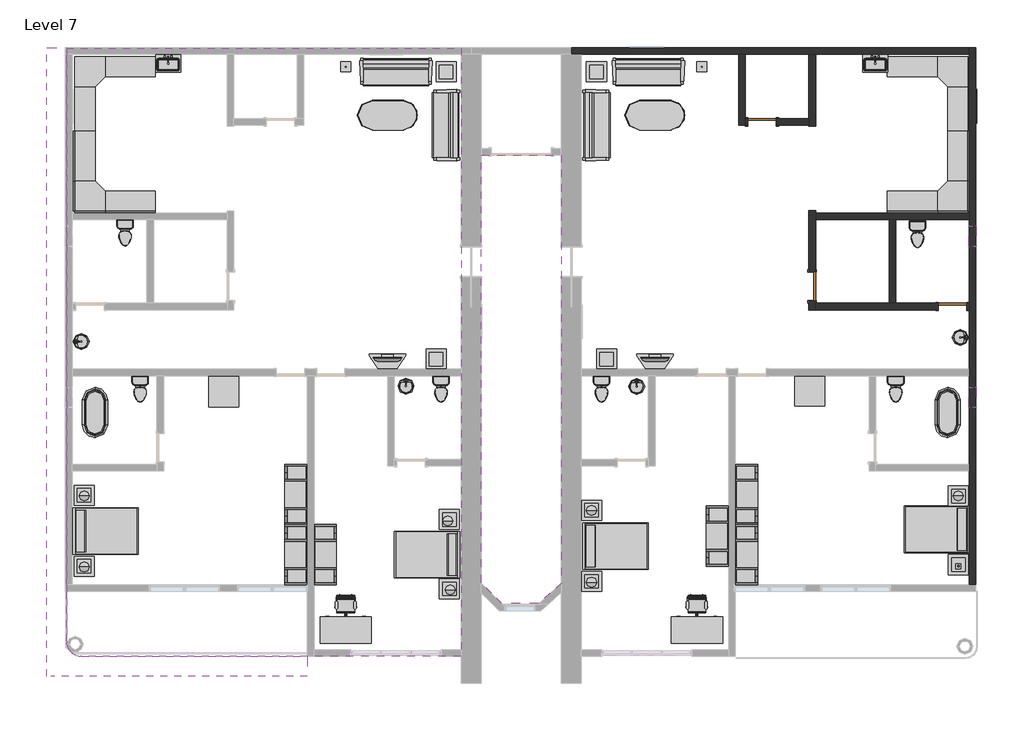
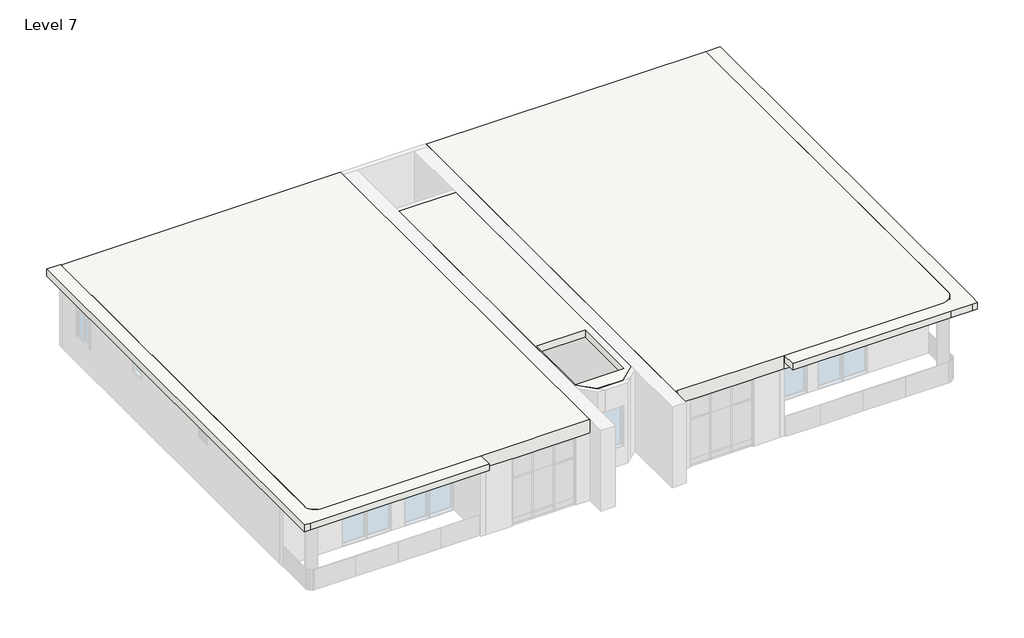
# One storey, part 3 of 3: 42 furniture elements, 14 flow terminals, 10 light fixtures, 9 walls, 3 doors, 3 slabs, 3 windows.
# Revit data of these elements (continued)
# Elements 40, 41 (IfcFurniture, "TV Stand : TV Stand") (continued)
#   Phase Created = New Construction
#   Materials on its faces: "Melamine - Gray", "Glass - Shelves"
# Elements 42, 43, 44, 45, 46, 47, 48, 49, 50, 51, 52, 53 (IfcFurniture, "Table-Coffee : 24\" x 24\" x 24\"")
#   Phase Created = New Construction
#   Materials on its faces: "Glass - Clear, Grey"
# Elements 54, 55 (IfcFurniture, "Table-Dining Oval : 36\" x 72\"")
#   Phase Created = New Construction
#   Materials on its faces: "Steel, Chrome Plated", "Glass - Clear, Grey"
# Elements 56, 57 (IfcFurniture, "Table-Rectangular : 36\" x 36\"")
#   Phase Created = New Construction
#   Materials on its faces: "Birch"
# Elements 58, 59 (IfcFurniture, "Work Station Cubicle : 96\" x 96\"")
#   Phase Created = New Construction
#   Materials on its faces: "Textile - Light Gray", "Laminate, Ivory, Matte"
# Element 60 (IfcLightFixture, "100W - 120V")
#   Mark = "84"
#   Phase Created = New Construction
#   Materials on its faces: "Steel, Chrome Plated", "Glass, Frosted"
# Element 61 (IfcLightFixture, "100W - 120V")
#   Mark = "85"
#   Phase Created = New Construction
#   Materials on its faces: "Steel, Chrome Plated", "Glass, Frosted"
# Element 62 (IfcLightFixture, "Table Lamp - Hemispheric : 60W - 120V")
#   Mark = "86"
#   Phase Created = New Construction
#   Materials on its faces: "Steel, Chrome Plated", "Glass, Frosted", "Birch"
# Element 63 (IfcLightFixture, "Table Lamp - Hemispheric : 60W - 120V")
#   Mark = "87"
#   Phase Created = New Construction
#   Materials on its faces: "Steel, Chrome Plated", "Glass, Frosted", "Birch"
# Element 64 (IfcLightFixture, "Table Lamp - Hemispheric : 60W - 120V")
#   Mark = "88"
#   Phase Created = New Construction
#   Materials on its faces: "Steel, Chrome Plated", "Glass, Frosted", "Birch"
# Element 65 (IfcLightFixture, "Table Lamp - Hemispheric : 60W - 120V")
#   Mark = "89"
#   Phase Created = New Construction
#   Materials on its faces: "Steel, Chrome Plated", "Glass, Frosted", "Birch"
# Element 66 (IfcLightFixture, "Table Lamp - Hemispheric : 60W - 120V")
#   Mark = "90"
#   Phase Created = New Construction
#   Materials on its faces: "Steel, Chrome Plated", "Glass, Frosted", "Birch"
# Element 67 (IfcLightFixture, "Table Lamp - Hemispheric : 60W - 120V")
#   Mark = "91"
#   Phase Created = New Construction
#   Materials on its faces: "Steel, Chrome Plated", "Glass, Frosted", "Birch"
# Element 68 (IfcLightFixture, "Table Lamp - Hemispheric : 60W - 120V")
#   Mark = "92"
#   Phase Created = New Construction
#   Materials on its faces: "Steel, Chrome Plated", "Glass, Frosted", "Birch"
# Element 69 (IfcLightFixture, "Table Lamp - Hemispheric : 60W - 120V")
#   Mark = "93"
#   Phase Created = New Construction
#   Materials on its faces: "Steel, Chrome Plated", "Glass, Frosted", "Birch"
# Element 70 (IfcSlab, "Generic - 12\" cream")
#   Height Offset From Level = 12' - 0"
#   Phase Created = New Construction
#   Materials on its faces: "Parking Stripe"
# Element 71 (IfcSlab, "Generic - 12\" white")
#   built-in parameter 1001955 = 3.14159 (stored number, unit not read)
#   Height Offset From Level = 12' - 0"
#   Phase Created = New Construction
#   Materials on its faces: "Door - Frame"
# Element 72 (IfcSlab, "Generic - 12\" white")
#   Height Offset From Level = 12' - 0"
#   Phase Created = New Construction
#   Materials on its faces: "Door - Frame"
# Elements 73, 74, 75, 76, 77, 78, 79, 80 (IfcWall, "Generic - 8\" cream")
#   Top Offset = 0' - 0"
#   Base Offset = 0' - 0"
#   Unconnected Height = 10' - 0"
#   wall height = 10' - 0"
#   Phase Created = New Construction
#   Base Constraint = Level 7
#   Materials on its faces: "Parking Stripe"
# Element 81 (IfcWall, "Generic - 8\" white")
#   Top Offset = 0' - 0"
#   Base Offset = 0' - 0"
#   Unconnected Height = 10' - 0"
#   wall height = 10' - 0"
#   Phase Created = New Construction
#   Base Constraint = Level 7
#   Materials on its faces: "Door - Frame", "Parking Stripe"
# Element 82 (IfcWindow, "Louvers with Trim : 24\" x 24\"")
#   Mark = "167"
#   Phase Created = New Construction
#   Materials on its faces: "Glass", "Iron, Ductile"
# Element 83 (IfcWindow, "Louvers with Trim : 24\" x 24\"")
#   Mark = "168"
#   Phase Created = New Construction
#   Materials on its faces: "Glass", "Iron, Ductile"
# Element 84 (IfcWindow, "Slider with Trim : 36\" x 48\"")
#   Mark = "164"
#   Phase Created = New Construction
#   Materials on its faces: "Iron, Ductile", "Glass"
# Materials
#   "Wood - Birch - Solid Stained Light Low Gloss": class "Wood", colour RGB 210 159 95, transparency 0, Cost = 0
#   "Paint - Sienna": colour RGB 118 70 51, transparency 0, Cost = 0
#   "Steel, Polished": class "Metal", colour RGB 57 57 57, transparency 0, Description = "Polished steel", Cost = 0
#   "Porcelain, Linen": class "Ceramic", colour RGB 249 239 230, transparency 0, Description = "Porcelain, linen", Cost = 0
#   "Laminate, Linen, Matte": class "Plastic", colour RGB 249 239 230, transparency 0, Description = "Plastic Laminate - Linen, Matte", Cost = 0
#   "Porcelain, Ivory": class "Ceramic", colour RGB 247 247 239, transparency 0, Description = "Porcelain, ivory", Cost = 0
#   "Laminate, Ivory, Matte": class "Plastic", colour RGB 247 247 239, transparency 0, Description = "Plastic Laminate - Ivory, Matte", Cost = 0
#   "Birch": class "Wood", colour RGB 224 178 126, transparency 0, Description = "Betula Alleghaniensis", Cost = 0
#   "Linen, White": class "Textile", colour RGB 247 247 239, transparency 0, Description = "Linen, white", Cost = 0
#   "Plastic, Opaque Black": class "Plastic", colour RGB 0 0 0, transparency 0.7, Description = "Plastic, generic, opaque black", Cost = 0
#   "Textile - Slate Blue": class "Fabric", colour RGB 98 102 118, transparency 0
#   "Steel, Chrome Plated": class "Metal", colour RGB 17 17 17, transparency 0, Description = "Chromiuim plated steel", Cost = 0
#   "Cherry": class "Wood", colour RGB 226 177 128, transparency 0, Description = "Prunus Serotina", Cost = 0
#   "Linen, Beige": class "Textile", colour RGB 249 239 230, transparency 0, Description = "Linen, beige", Cost = 0
#   "Melamine - Gray": class "Wood", colour RGB 49 49 49, transparency 0
#   "Glass - Clear, Grey": class "Glass", colour RGB 252 255 255, transparency 0.64
#   "Textile - Light Gray": class "Fabric", colour RGB 204 204 204, transparency 0
#   "Glass, Frosted": class "Glass", colour RGB 250 244 225, transparency 0.55, Description = "physical material", Cost = 0
#   "Parking Stripe": class "Paint", colour RGB 250 250 91, transparency 0, Cost = 0
#   "Door - Frame": colour RGB 118 70 51, transparency 0, Cost = 0
#   "Iron, Ductile": class "Metal", colour RGB 0 0 0, transparency 0, Description = "Ductile cast iron", Cost = 0
#   "Glass": class "Glass", colour RGB 0 128 192, transparency 0.75, Description = "Soda Lime Glass", Cost = 0
#   "TV - Black": colour RGB 49 49 49, transparency 0
#   "TV - Glass": colour RGB 157 157 157, transparency 0.9
#   "TV - Screen": colour RGB 0 0 0, transparency 0
#   "Glass - Shelves": class "Glass", colour RGB 167 167 167, transparency 0.9
